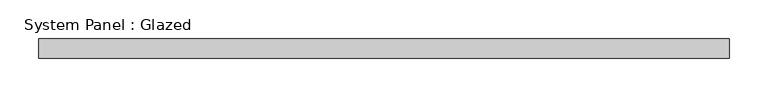
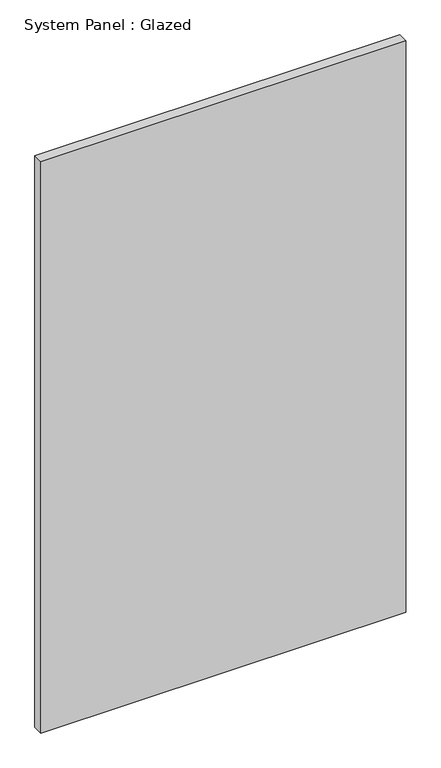
"""IFC4 building model written with IfcOpenShell, lengths in millimetres: plate geometry, System Panel : Glazed."""

from ifc_helpers import new_model, si_unit, origin, origin_with_axes, place, context, project, spatial, polyline, outline, extrude, source, transform, mapped, element, save


def system_panel_glazed_d3edc084(model_context):
    return source(origin(), model_context, "Body", "SweptSolid", [
        extrude(outline(polyline([(447.675, 19.05), (-447.675, 19.05), (-447.675, 44.45), (447.675, 44.45), (447.675, 19.05)])), origin_with_axes(), (0.0, 0.0, 1.0), 1482.522501),
    ])


if __name__ == "__main__":
    model = new_model("IFC4")
    model_context = context("Model", 3, world=origin())
    ifc_project = project(units=[si_unit("LENGTHUNIT", "METRE", prefix="MILLI")], contexts=[model_context])
    site = spatial("IfcSite", under=ifc_project)
    building = spatial("IfcBuilding", under=site)
    placement = place(None, origin())
    system_panel_glazed_shape = system_panel_glazed_d3edc084(model_context)
    element("IfcPlate", 1, ObjectType="System Panel : Glazed", at=placement, inside=building, context=model_context, shape_type="MappedRepresentation", body=[
        mapped(system_panel_glazed_shape, transform((0.0, 0.0, 0.0), x_axis=(1.0, 0.0, 0.0), y_axis=(0.0, 1.0, 0.0), z_axis=(0.0, 0.0, 1.0))),
    ])
    save(model, "model.ifc")

# Revit data of these elements
# Type "System Panel : Glazed"
#   Construction Type Id = "GSP4R"
#   Analytic Construction = "1/8 in Pilkington single glazing"
#   Visual Light Transmittance = 0.9
#   Solar Heat Gain Coefficient = 0.86
#   Heat Transfer Coefficient (U) = 1.18115 BTU/(h·ft²·°F)
#   Define Thermal Properties by = 1
# Element 1 (IfcPlate, "System Panel : Glazed")
#   Materials on its faces: "Glass"
# Materials
#   "Glass": class "Glass", colour RGB 0 128 192, transparency 0.75, Description = "Soda Lime Glass", Cost = 0
